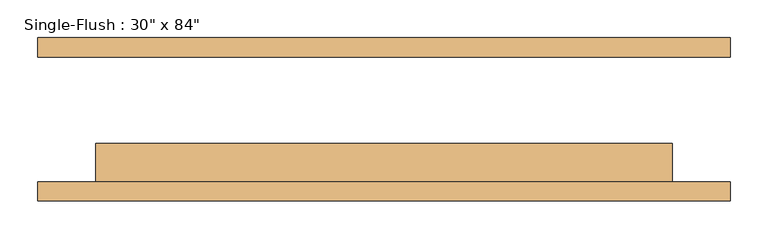
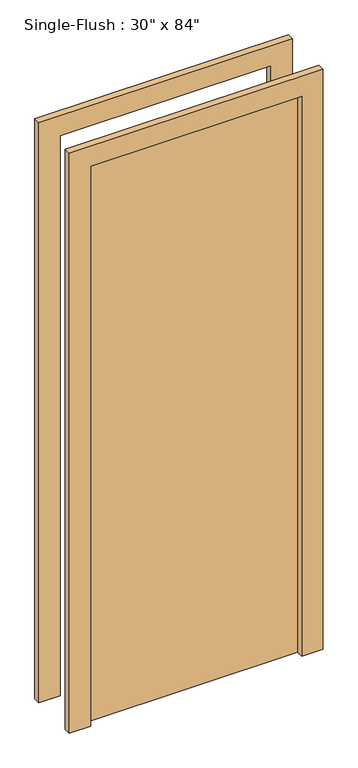
"""IFC4 building model written with IfcOpenShell, lengths in millimetres: door geometry."""

from ifc_helpers import new_model, si_unit, frame, origin, origin_with_axes, place, context, project, spatial, polyline, outline, extrude, source, transform, mapped, element, save


def door_3dc6c820(model_context):
    return source(origin(), model_context, "Body", "SweptSolid", [
        extrude(outline(polyline([(2209.8, -457.2), (0.0, -457.2), (0.0, -381.0), (2133.6, -381.0), (2133.6, 381.0), (0.0, 381.0), (0.0, 457.2), (2209.8, 457.2), (2209.8, -457.2)])), frame((0.0, -107.95, 0.0), z_axis=(0.0, 1.0, 0.0), x_axis=(0.0, 0.0, 1.0)), (0.0, 0.0, 1.0), 25.4),
        extrude(outline(polyline([(2209.8, 457.2), (2209.8, -457.2), (0.0, -457.2), (0.0, -381.0), (2133.6, -381.0), (2133.6, 381.0), (0.0, 381.0), (0.0, 457.2), (2209.8, 457.2)])), frame((0.0, 82.55, 0.0), z_axis=(0.0, 1.0, 0.0), x_axis=(0.0, 0.0, 1.0)), (0.0, 0.0, 1.0), 25.4),
        extrude(outline(polyline([(381.0, -31.75), (381.0, -82.55), (-381.0, -82.55), (-381.0, -31.75), (381.0, -31.75)])), origin_with_axes(), (0.0, 0.0, 1.0), 2133.6),
    ])


if __name__ == "__main__":
    model = new_model("IFC4")
    model_context = context("Model", 3, world=origin())
    ifc_project = project(units=[si_unit("LENGTHUNIT", "METRE", prefix="MILLI")], contexts=[model_context])
    site = spatial("IfcSite", under=ifc_project)
    building = spatial("IfcBuilding", under=site)
    placement = place(None, origin())
    door_shape = door_3dc6c820(model_context)
    element("IfcDoor", 1, ObjectType="Single-Flush : 30\" x 84\"", at=placement, inside=building, context=model_context, shape_type="MappedRepresentation", body=[
        mapped(door_shape, transform((0.0, 0.0, 0.0), x_axis=(1.0, 0.0, 0.0), y_axis=(0.0, 1.0, 0.0), z_axis=(0.0, 0.0, 1.0))),
    ])
    save(model, "model.ifc")

# Revit data of these elements
# Type "Single-Flush : 30\" x 84\""
#   Type Mark = "4"
#   Construction Type Id = "MDOOR"
#   Assembly Code = "C1020"
#   Analytic Construction = "Metal"
#   Thickness = 0' - 2"
#   Heat Transfer Coefficient (U) = 0.651978 BTU/(h·ft²·°F)
#   Height = 7' - 0"
#   Trim Projection Ext = 0' - 1"
#   Trim Projection Int = 0' - 1"
#   Trim Width = 0' - 3"
#   Width = 2' - 6"
#   Define Thermal Properties by = 1
#   Define Thermal Properties by = 1
#   Door Material = Door - Panel
#   Frame Material = Door - Frame
#   Visual Light Transmittance = 0
#   Solar Heat Gain Coefficient = 0
#   Function = (empty or 0)
#   Wall Closure = (empty or 0)
# Element 1 (IfcDoor, "Single-Flush : 30\" x 84\"")
#   Materials on its faces: "Door - Frame", "Door - Panel"
# Materials
#   "Door - Panel": class "Wood", colour RGB 210 159 95, transparency 0, Cost = 0
#   "Door - Frame": colour RGB 118 70 51, transparency 0, Cost = 0
